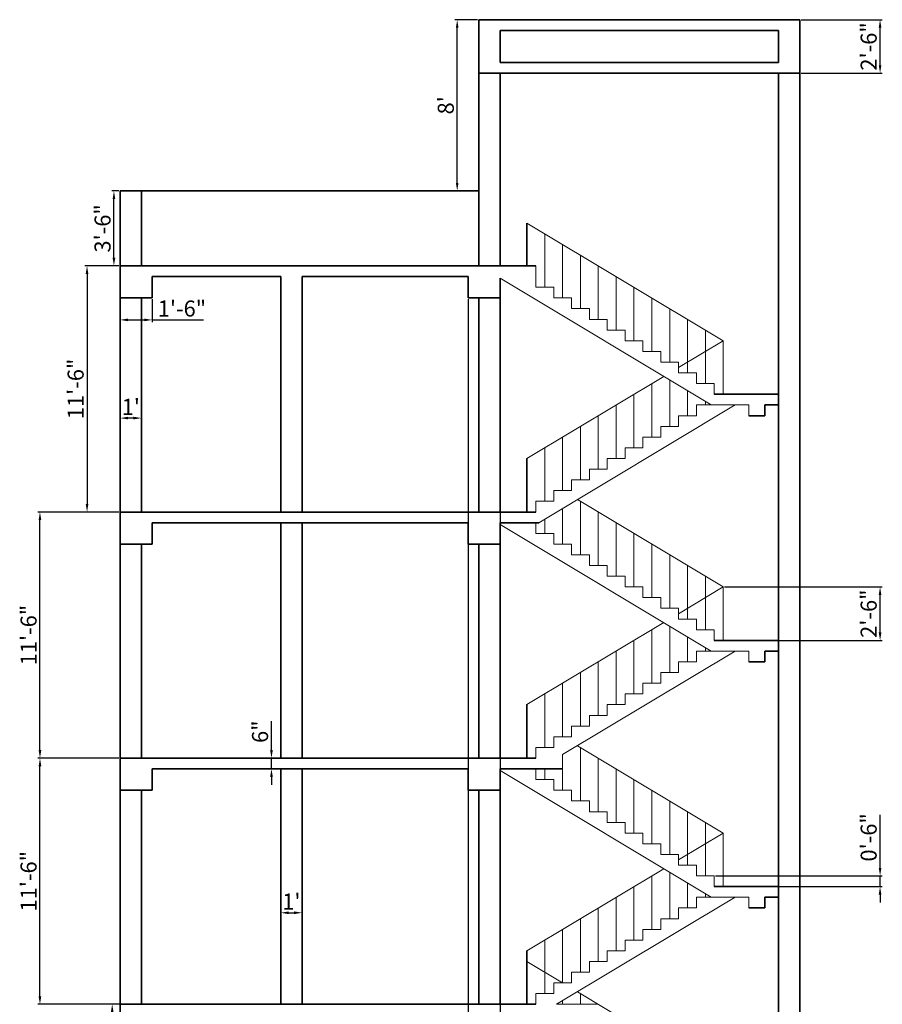
# Model space of a CAD drawing. Units: inches. Extents: x 1692 to 2762, y 798 to 1757.
# Tile 4 of 4: x 2279 to 2762, y 1156 to 1708. Entities that reach past the tile are written whole.
import ezdxf

# ---------------------------------------------------------------- set-up
doc = ezdxf.new("R2010")
doc.units = ezdxf.units.IN
for name, color, linetype, lineweight in [('A-ANNO-DIMS', 2, 'Continuous', 18), ('A-FLOR-STRS', 3, 'Continuous', 18), ('A-SECT', 1, 'Continuous', 35)]:
    doc.layers.add(name, color=color, linetype=linetype, lineweight=lineweight)
doc.styles.get("Standard").update_dxf_attribs({"font": 'arial.ttf'})
doc.dimstyles.new('ISO-25', dxfattribs={"dimtxt": 9, "dimasz": 4.5, "dimexe": 1.25, "dimexo": 0.625, "dimtad": 1, "dimdec": 0, "dimlunit": 3, "dimtxsty": 'Standard', "dimcen": 2.5, "dimadec": 0, "dimazin": 0, "dimtfac": 1, "dimtdec": 0, "dimtmove": 0, "dimatfit": 3, "dimfxl": 1, "dimarcsym": 0})

# ---------------------------------------------------------------- blocks, each defined once
blk = doc.blocks.new('*D1')
at = {"layer": 'A-ANNO-DIMS', "color": 0, "lineweight": -2, "transparency": 16777216}
for p, q in [((2334.16, 1570.43), (2315.01, 1570.43)), ((2316.26, 1565.93), (2316.26, 1436.93)), ((2334.16, 1432.43), (2315.01, 1432.43))]:
    blk.add_line(p, q, dxfattribs=at)
at = {"layer": 'A-ANNO-DIMS', "color": 0, "lineweight": 0, "transparency": 16777216}
for points in [[(2315.51, 1565.93), (2317.01, 1565.93), (2316.26, 1570.43)], [(2315.51, 1436.93), (2317.01, 1436.93), (2316.26, 1432.43)]]:
    blk.add_solid(points, dxfattribs=at)
at = {"layer": 'Defpoints', "color": 0, "lineweight": 0, "transparency": 16777216}
for p in [(2334.78, 1570.43), (2316.26, 1432.43), (2334.78, 1432.43)]:
    blk.add_point(p, dxfattribs=at)
at = {"layer": 'A-ANNO-DIMS', "color": 0, "transparency": 16777216, "insert": (2311.04, 1501.43), "char_height": 9, "attachment_point": 5, "rotation": 90}
blk.add_mtext('11\'-6"', dxfattribs=at)
blk = doc.blocks.new('*D2')
at = {"layer": 'A-ANNO-DIMS', "color": 0, "lineweight": -2, "transparency": 16777216}
for p, q in [((2334.78, 1551.81), (2334.78, 1538.88)), ((2352.78, 1551.81), (2352.78, 1538.88)), ((2339.28, 1540.13), (2348.28, 1540.13)), ((2352.78, 1540.13), (2381.61, 1540.13))]:
    blk.add_line(p, q, dxfattribs=at)
at = {"layer": 'A-ANNO-DIMS', "color": 0, "lineweight": 0, "transparency": 16777216}
for points in [[(2339.28, 1540.88), (2339.28, 1539.38), (2334.78, 1540.13)], [(2348.28, 1540.88), (2348.28, 1539.38), (2352.78, 1540.13)]]:
    blk.add_solid(points, dxfattribs=at)
at = {"layer": 'Defpoints', "color": 0, "lineweight": 0, "transparency": 16777216}
for p in [(2334.78, 1552.43), (2352.78, 1552.43), (2352.78, 1540.13)]:
    blk.add_point(p, dxfattribs=at)
at = {"layer": 'A-ANNO-DIMS', "color": 0, "transparency": 16777216, "insert": (2369.44, 1545.35), "char_height": 9, "attachment_point": 5}
blk.add_mtext('1\'-6"', dxfattribs=at)
blk = doc.blocks.new('*D3')
at = {"layer": 'A-ANNO-DIMS', "color": 0, "lineweight": -2, "transparency": 16777216}
for p, q in [((2334.78, 1478.04), (2334.78, 1486.33)), ((2342.28, 1485.08), (2339.28, 1485.08)), ((2346.78, 1478.04), (2346.78, 1486.33))]:
    blk.add_line(p, q, dxfattribs=at)
at = {"layer": 'A-ANNO-DIMS', "color": 0, "lineweight": 0, "transparency": 16777216}
for points in [[(2339.28, 1485.83), (2339.28, 1484.33), (2334.78, 1485.08)], [(2342.28, 1485.83), (2342.28, 1484.33), (2346.78, 1485.08)]]:
    blk.add_solid(points, dxfattribs=at)
at = {"layer": 'Defpoints', "color": 0, "lineweight": 0, "transparency": 16777216}
for p in [(2334.78, 1485.08), (2334.78, 1477.42), (2346.78, 1477.42)]:
    blk.add_point(p, dxfattribs=at)
at = {"layer": 'A-ANNO-DIMS', "color": 0, "transparency": 16777216, "insert": (2340.78, 1490.22), "char_height": 9, "attachment_point": 5}
blk.add_mtext("1'", dxfattribs=at)
blk = doc.blocks.new('*D5')
at = {"layer": 'A-ANNO-DIMS', "color": 0, "lineweight": -2, "transparency": 16777216}
for p, q in [((2346.16, 1156.43), (2329.11, 1156.43)), ((2330.36, 1151.93), (2330.36, 1142.93)), ((2346.16, 1138.43), (2329.11, 1138.43)), ((2330.36, 1138.43), (2330.36, 1109.61))]:
    blk.add_line(p, q, dxfattribs=at)
at = {"layer": 'A-ANNO-DIMS', "color": 0, "lineweight": 0, "transparency": 16777216}
for points in [[(2329.61, 1151.93), (2331.11, 1151.93), (2330.36, 1156.43)], [(2329.61, 1142.93), (2331.11, 1142.93), (2330.36, 1138.43)]]:
    blk.add_solid(points, dxfattribs=at)
at = {"layer": 'Defpoints', "color": 0, "lineweight": 0, "transparency": 16777216}
for p in [(2346.78, 1156.43), (2330.36, 1138.43), (2346.78, 1138.43)]:
    blk.add_point(p, dxfattribs=at)
at = {"layer": 'A-ANNO-DIMS', "color": 0, "transparency": 16777216, "insert": (2325.14, 1121.77), "char_height": 9, "attachment_point": 5, "rotation": 90}
blk.add_mtext('1\'-6"', dxfattribs=at)
blk = doc.blocks.new('*D7')
at = {"layer": 'A-ANNO-DIMS', "color": 0, "lineweight": -2, "transparency": 16777216}
for p, q in [((2424.78, 1195.02), (2424.78, 1209.01)), ((2436.78, 1195.02), (2436.78, 1209.01)), ((2429.28, 1207.76), (2432.28, 1207.76))]:
    blk.add_line(p, q, dxfattribs=at)
at = {"layer": 'A-ANNO-DIMS', "color": 0, "lineweight": 0, "transparency": 16777216}
for points in [[(2429.28, 1208.51), (2429.28, 1207.01), (2424.78, 1207.76)], [(2432.28, 1208.51), (2432.28, 1207.01), (2436.78, 1207.76)]]:
    blk.add_solid(points, dxfattribs=at)
at = {"layer": 'Defpoints', "color": 0, "lineweight": 0, "transparency": 16777216}
for p in [(2436.78, 1207.76), (2424.78, 1194.4), (2436.78, 1194.4)]:
    blk.add_point(p, dxfattribs=at)
at = {"layer": 'A-ANNO-DIMS', "color": 0, "transparency": 16777216, "insert": (2430.78, 1212.9), "char_height": 9, "attachment_point": 5}
blk.add_mtext("1'", dxfattribs=at)
blk = doc.blocks.new('*D8')
at = {"layer": 'A-ANNO-DIMS', "color": 0, "lineweight": -2, "transparency": 16777216}
for p, q in [((2419.61, 1298.93), (2419.61, 1315.08)), ((2417.71, 1294.43), (2420.86, 1294.43)), ((2419.61, 1288.43), (2419.61, 1294.43)), ((2417.71, 1288.43), (2420.86, 1288.43)), ((2419.61, 1283.93), (2419.61, 1279.43))]:
    blk.add_line(p, q, dxfattribs=at)
at = {"layer": 'A-ANNO-DIMS', "color": 0, "lineweight": 0, "transparency": 16777216}
for points in [[(2418.86, 1298.93), (2420.36, 1298.93), (2419.61, 1294.43)], [(2418.86, 1283.93), (2420.36, 1283.93), (2419.61, 1288.43)]]:
    blk.add_solid(points, dxfattribs=at)
at = {"layer": 'Defpoints', "color": 0, "lineweight": 0, "transparency": 16777216}
for p in [(2417.08, 1294.43), (2419.61, 1294.43), (2417.08, 1288.43)]:
    blk.add_point(p, dxfattribs=at)
at = {"layer": 'A-ANNO-DIMS', "color": 0, "transparency": 16777216, "insert": (2414.39, 1309.25), "char_height": 9, "attachment_point": 5, "rotation": 90}
blk.add_mtext('6"', dxfattribs=at)
blk = doc.blocks.new('*D9')
at = {"layer": 'A-ANNO-DIMS', "color": 0, "lineweight": -2, "transparency": 16777216}
for p, q in [((2334.16, 1612.43), (2330.09, 1612.43)), ((2331.34, 1574.93), (2331.34, 1607.93)), ((2334.16, 1570.43), (2330.09, 1570.43))]:
    blk.add_line(p, q, dxfattribs=at)
at = {"layer": 'A-ANNO-DIMS', "color": 0, "lineweight": 0, "transparency": 16777216}
for points in [[(2330.59, 1607.93), (2332.09, 1607.93), (2331.34, 1612.43)], [(2330.59, 1574.93), (2332.09, 1574.93), (2331.34, 1570.43)]]:
    blk.add_solid(points, dxfattribs=at)
at = {"layer": 'Defpoints', "color": 0, "lineweight": 0, "transparency": 16777216}
for p in [(2331.34, 1612.43), (2334.78, 1612.43), (2334.78, 1570.43)]:
    blk.add_point(p, dxfattribs=at)
at = {"layer": 'A-ANNO-DIMS', "color": 0, "transparency": 16777216, "insert": (2326.12, 1591.43), "char_height": 9, "attachment_point": 5, "rotation": 90}
blk.add_mtext('3\'-6"', dxfattribs=at)
blk = doc.blocks.new('*D10')
at = {"layer": 'A-ANNO-DIMS', "color": 0, "lineweight": -2, "transparency": 16777216}
for p, q in [((2535.16, 1708.43), (2522.45, 1708.43)), ((2523.7, 1616.93), (2523.7, 1703.93)), ((2535.16, 1612.43), (2522.45, 1612.43))]:
    blk.add_line(p, q, dxfattribs=at)
at = {"layer": 'A-ANNO-DIMS', "color": 0, "lineweight": 0, "transparency": 16777216}
for points in [[(2522.95, 1703.93), (2524.45, 1703.93), (2523.7, 1708.43)], [(2522.95, 1616.93), (2524.45, 1616.93), (2523.7, 1612.43)]]:
    blk.add_solid(points, dxfattribs=at)
at = {"layer": 'Defpoints', "color": 0, "lineweight": 0, "transparency": 16777216}
for p in [(2523.7, 1708.43), (2535.78, 1708.43), (2535.78, 1612.43)]:
    blk.add_point(p, dxfattribs=at)
at = {"layer": 'A-ANNO-DIMS', "color": 0, "transparency": 16777216, "insert": (2518.48, 1660.43), "char_height": 9, "attachment_point": 5, "rotation": 90}
blk.add_mtext("8'", dxfattribs=at)
blk = doc.blocks.new('*D54')
at = {"layer": 'A-ANNO-DIMS', "color": 0, "lineweight": -2, "transparency": 16777216}
for p, q in [((2334.16, 1294.43), (2288.63, 1294.43)), ((2289.88, 1160.93), (2289.88, 1289.93)), ((2334.16, 1156.43), (2288.63, 1156.43))]:
    blk.add_line(p, q, dxfattribs=at)
at = {"layer": 'A-ANNO-DIMS', "color": 0, "lineweight": 0, "transparency": 16777216}
for points in [[(2289.13, 1289.93), (2290.63, 1289.93), (2289.88, 1294.43)], [(2289.13, 1160.93), (2290.63, 1160.93), (2289.88, 1156.43)]]:
    blk.add_solid(points, dxfattribs=at)
at = {"layer": 'Defpoints', "color": 0, "lineweight": 0, "transparency": 16777216}
for p in [(2289.88, 1294.43), (2334.78, 1294.43), (2334.78, 1156.43)]:
    blk.add_point(p, dxfattribs=at)
at = {"layer": 'A-ANNO-DIMS', "color": 0, "transparency": 16777216, "insert": (2284.66, 1225.43), "char_height": 9, "attachment_point": 5, "rotation": 90}
blk.add_mtext('11\'-6"', dxfattribs=at)
blk = doc.blocks.new('*D55')
at = {"layer": 'A-ANNO-DIMS', "color": 0, "lineweight": -2, "transparency": 16777216}
for p, q in [((2334.16, 1432.43), (2288.63, 1432.43)), ((2289.88, 1298.93), (2289.88, 1427.93)), ((2334.16, 1294.43), (2288.63, 1294.43))]:
    blk.add_line(p, q, dxfattribs=at)
at = {"layer": 'A-ANNO-DIMS', "color": 0, "lineweight": 0, "transparency": 16777216}
for points in [[(2289.13, 1427.93), (2290.63, 1427.93), (2289.88, 1432.43)], [(2289.13, 1298.93), (2290.63, 1298.93), (2289.88, 1294.43)]]:
    blk.add_solid(points, dxfattribs=at)
at = {"layer": 'Defpoints', "color": 0, "lineweight": 0, "transparency": 16777216}
for p in [(2289.88, 1432.43), (2334.78, 1432.43), (2334.78, 1294.43)]:
    blk.add_point(p, dxfattribs=at)
at = {"layer": 'A-ANNO-DIMS', "color": 0, "transparency": 16777216, "insert": (2284.66, 1363.43), "char_height": 9, "attachment_point": 5, "rotation": 90}
blk.add_mtext('11\'-6"', dxfattribs=at)
blk = doc.blocks.new('*D56')
at = {"layer": 'A-ANNO-DIMS', "color": 0, "lineweight": -2, "transparency": 16777216}
for p, q in [((2716.41, 1708.43), (2761.93, 1708.43)), ((2760.68, 1682.93), (2760.68, 1703.93)), ((2716.41, 1678.43), (2761.93, 1678.43))]:
    blk.add_line(p, q, dxfattribs=at)
at = {"layer": 'A-ANNO-DIMS', "color": 0, "lineweight": 0, "transparency": 16777216}
for points in [[(2759.93, 1703.93), (2761.43, 1703.93), (2760.68, 1708.43)], [(2759.93, 1682.93), (2761.43, 1682.93), (2760.68, 1678.43)]]:
    blk.add_solid(points, dxfattribs=at)
at = {"layer": 'Defpoints', "color": 0, "lineweight": 0, "transparency": 16777216}
for p in [(2715.78, 1708.43), (2760.68, 1708.43), (2715.78, 1678.43)]:
    blk.add_point(p, dxfattribs=at)
at = {"layer": 'A-ANNO-DIMS', "color": 0, "transparency": 16777216, "insert": (2755.46, 1693.43), "char_height": 9, "attachment_point": 5, "rotation": 90}
blk.add_mtext('2\'-6"', dxfattribs=at)
blk = doc.blocks.new('*D65')
at = {"layer": 'A-ANNO-DIMS', "color": 0, "lineweight": -2, "transparency": 16777216}
for p, q in [((2529.78, 1551.81), (2529.78, 798.28)), ((2547.78, 1551.81), (2547.78, 798.28)), ((2534.28, 799.53), (2543.28, 799.53)), ((2547.78, 799.53), (2576.61, 799.53))]:
    blk.add_line(p, q, dxfattribs=at)
at = {"layer": 'A-ANNO-DIMS', "color": 0, "lineweight": 0, "transparency": 16777216}
for points in [[(2534.28, 800.28), (2534.28, 798.78), (2529.78, 799.53)], [(2543.28, 800.28), (2543.28, 798.78), (2547.78, 799.53)]]:
    blk.add_solid(points, dxfattribs=at)
at = {"layer": 'Defpoints', "color": 0, "lineweight": 0, "transparency": 16777216}
for p in [(2529.78, 1552.43), (2547.78, 1552.43), (2547.78, 799.53)]:
    blk.add_point(p, dxfattribs=at)
at = {"layer": 'A-ANNO-DIMS', "color": 0, "transparency": 16777216, "insert": (2564.44, 804.75), "char_height": 9, "attachment_point": 5}
blk.add_mtext('1\'-6"', dxfattribs=at)
blk = doc.blocks.new('*D67')
at = {"layer": 'A-ANNO-DIMS', "color": 0, "lineweight": -2, "transparency": 16777216}
for p, q in [((2760.68, 1232.93), (2760.68, 1262.61)), ((2668.41, 1228.43), (2761.93, 1228.43)), ((2760.68, 1222.43), (2760.68, 1228.43)), ((2668.41, 1222.43), (2761.93, 1222.43)), ((2760.68, 1217.93), (2760.68, 1213.43))]:
    blk.add_line(p, q, dxfattribs=at)
at = {"layer": 'A-ANNO-DIMS', "color": 0, "lineweight": 0, "transparency": 16777216}
for points in [[(2759.93, 1232.93), (2761.43, 1232.93), (2760.68, 1228.43)], [(2759.93, 1217.93), (2761.43, 1217.93), (2760.68, 1222.43)]]:
    blk.add_solid(points, dxfattribs=at)
at = {"layer": 'Defpoints', "color": 0, "lineweight": 0, "transparency": 16777216}
for p in [(2667.78, 1228.43), (2760.68, 1228.43), (2667.78, 1222.43)]:
    blk.add_point(p, dxfattribs=at)
at = {"layer": 'A-ANNO-DIMS', "color": 0, "transparency": 16777216, "insert": (2755.46, 1250.02), "char_height": 9, "attachment_point": 5, "rotation": 90}
blk.add_mtext('0\'-6"', dxfattribs=at)
blk = doc.blocks.new('*D68')
at = {"layer": 'A-ANNO-DIMS', "color": 0, "lineweight": -2, "transparency": 16777216}
for p, q in [((2673.41, 1390.43), (2761.93, 1390.43)), ((2760.68, 1364.93), (2760.68, 1385.93)), ((2673.41, 1360.43), (2761.93, 1360.43))]:
    blk.add_line(p, q, dxfattribs=at)
at = {"layer": 'A-ANNO-DIMS', "color": 0, "lineweight": 0, "transparency": 16777216}
for points in [[(2759.93, 1385.93), (2761.43, 1385.93), (2760.68, 1390.43)], [(2759.93, 1364.93), (2761.43, 1364.93), (2760.68, 1360.43)]]:
    blk.add_solid(points, dxfattribs=at)
at = {"layer": 'Defpoints', "color": 0, "lineweight": 0, "transparency": 16777216}
for p in [(2672.78, 1390.43), (2760.68, 1390.43), (2672.78, 1360.43)]:
    blk.add_point(p, dxfattribs=at)
at = {"layer": 'A-ANNO-DIMS', "color": 0, "transparency": 16777216, "insert": (2755.46, 1375.43), "char_height": 9, "attachment_point": 5, "rotation": 90}
blk.add_mtext('2\'-6"', dxfattribs=at)

msp = doc.modelspace()

# ---------------------------------------------------------------- linework, layer by layer
at = {"layer": 'A-FLOR-STRS'}
for p, q in [((2562.78, 1594.43), (2672.78, 1528.43)), ((2572.78, 1558.43), (2572.78, 1588.43)), ((2582.78, 1552.43), (2582.78, 1582.43)), ((2592.78, 1546.43), (2592.78, 1576.43)), ((2567.78, 1558.43), (2567.78, 1570.43)), ((2602.78, 1540.43), (2602.78, 1570.43)), ((2666.12, 1492.43), (2547.78, 1563.44)), ((2612.78, 1534.43), (2612.78, 1564.43)), ((2577.78, 1558.43), (2567.78, 1558.43)), ((2577.78, 1552.43), (2577.78, 1558.43)), ((2622.78, 1528.43), (2622.78, 1558.43)), ((2587.78, 1552.43), (2577.78, 1552.43)), ((2587.78, 1546.43), (2587.78, 1552.43)), ((2632.78, 1522.43), (2632.78, 1552.43)), ((2597.78, 1546.43), (2587.78, 1546.43)), ((2597.78, 1540.43), (2597.78, 1546.43)), ((2642.78, 1516.43), (2642.78, 1546.43)), ((2607.78, 1540.43), (2597.78, 1540.43)), ((2607.78, 1534.43), (2607.78, 1540.43)), ((2652.78, 1510.43), (2652.78, 1540.43)), ((2617.78, 1534.43), (2607.78, 1534.43)), ((2617.78, 1528.43), (2617.78, 1534.43)), ((2662.78, 1504.43), (2662.78, 1534.43)), ((2627.78, 1528.43), (2617.78, 1528.43)), ((2627.78, 1522.43), (2627.78, 1528.43)), ((2672.78, 1528.43), (2647.78, 1513.43)), ((2672.78, 1498.43), (2672.78, 1528.43)), ((2672.78, 1504.43), (2672.78, 1528.43)), ((2637.78, 1522.43), (2627.78, 1522.43)), ((2637.78, 1516.43), (2637.78, 1522.43)), ((2662.78, 1504.43), (2662.78, 1522.43)), ((2647.78, 1516.43), (2637.78, 1516.43)), ((2647.78, 1510.43), (2647.78, 1516.43)), ((2652.78, 1510.43), (2652.78, 1516.43)), ((2639.45, 1508.43), (2562.78, 1462.43)), ((2657.78, 1510.43), (2647.78, 1510.43)), ((2657.78, 1504.43), (2657.78, 1510.43)), ((2632.78, 1474.43), (2632.78, 1504.43)), ((2642.78, 1480.43), (2642.78, 1506.44)), ((2667.78, 1504.43), (2657.78, 1504.43)), ((2667.78, 1498.43), (2667.78, 1504.43)), ((2672.78, 1498.43), (2672.78, 1504.43)), ((2622.78, 1468.43), (2622.78, 1498.43)), ((2652.78, 1486.43), (2652.78, 1500.44)), ((2679.44, 1492.43), (2569.44, 1426.43)), ((2612.78, 1462.43), (2612.78, 1492.43)), ((2657.78, 1486.43), (2657.78, 1492.43)), ((2657.78, 1492.43), (2679.44, 1492.43)), ((2662.78, 1492.43), (2662.78, 1494.44)), ((2679.44, 1492.43), (2687.11, 1492.43)), ((2687.11, 1492.43), (2687.11, 1486.43)), ((2602.78, 1456.43), (2602.78, 1486.43)), ((2647.78, 1480.43), (2647.78, 1486.43)), ((2647.78, 1486.43), (2657.78, 1486.43)), ((2592.78, 1450.43), (2592.78, 1480.43)), ((2637.78, 1474.43), (2637.78, 1480.43)), ((2637.78, 1480.43), (2647.78, 1480.43)), ((2582.78, 1444.43), (2582.78, 1474.43)), ((2627.78, 1468.43), (2627.78, 1474.43)), ((2627.78, 1474.43), (2637.78, 1474.43)), ((2572.78, 1438.43), (2572.78, 1468.43)), ((2617.78, 1462.43), (2617.78, 1468.43)), ((2617.78, 1468.43), (2627.78, 1468.43)), ((2607.78, 1456.43), (2607.78, 1462.43)), ((2607.78, 1462.43), (2617.78, 1462.43)), ((2597.78, 1450.43), (2597.78, 1456.43)), ((2597.78, 1456.43), (2607.78, 1456.43)), ((2572.78, 1438.43), (2572.78, 1450.43)), ((2587.78, 1444.43), (2587.78, 1450.43)), ((2587.78, 1450.43), (2597.78, 1450.43)), ((2577.78, 1438.43), (2577.78, 1444.43)), ((2577.78, 1444.43), (2587.78, 1444.43)), ((2567.78, 1432.43), (2567.78, 1438.43)), ((2567.78, 1438.43), (2577.78, 1438.43)), ((2591.11, 1439.43), (2672.78, 1390.43)), ((2592.78, 1408.43), (2592.78, 1438.43)), ((2582.78, 1414.43), (2582.78, 1434.44)), ((2602.78, 1402.43), (2602.78, 1432.43)), ((2666.12, 1354.43), (2547.78, 1425.44)), ((2567.78, 1426.43), (2569.44, 1426.43)), ((2567.78, 1420.43), (2567.78, 1426.43)), ((2567.78, 1420.43), (2567.78, 1426.43)), ((2572.78, 1420.43), (2572.78, 1428.44)), ((2612.78, 1396.43), (2612.78, 1426.43)), ((2577.78, 1420.43), (2567.78, 1420.43)), ((2577.78, 1414.43), (2577.78, 1420.43)), ((2622.78, 1390.43), (2622.78, 1420.43)), ((2587.78, 1414.43), (2577.78, 1414.43)), ((2587.78, 1408.43), (2587.78, 1414.43)), ((2632.78, 1384.43), (2632.78, 1414.43)), ((2597.78, 1408.43), (2587.78, 1408.43)), ((2597.78, 1402.43), (2597.78, 1408.43)), ((2642.78, 1378.43), (2642.78, 1408.43)), ((2607.78, 1402.43), (2597.78, 1402.43)), ((2607.78, 1396.43), (2607.78, 1402.43)), ((2652.78, 1372.43), (2652.78, 1402.43)), ((2617.78, 1396.43), (2607.78, 1396.43)), ((2617.78, 1390.43), (2617.78, 1396.43)), ((2662.78, 1366.43), (2662.78, 1396.43)), ((2627.78, 1390.43), (2617.78, 1390.43)), ((2627.78, 1384.43), (2627.78, 1390.43)), ((2672.78, 1390.43), (2647.78, 1375.43)), ((2672.78, 1360.43), (2672.78, 1390.43)), ((2672.78, 1366.43), (2672.78, 1390.43)), ((2637.78, 1384.43), (2627.78, 1384.43)), ((2637.78, 1378.43), (2637.78, 1384.43)), ((2662.78, 1366.43), (2662.78, 1384.43)), ((2647.78, 1378.43), (2637.78, 1378.43)), ((2647.78, 1372.43), (2647.78, 1378.43)), ((2652.78, 1372.43), (2652.78, 1378.43)), ((2639.45, 1370.43), (2562.78, 1324.43)), ((2657.78, 1372.43), (2647.78, 1372.43)), ((2657.78, 1366.43), (2657.78, 1372.43)), ((2632.78, 1336.43), (2632.78, 1366.43)), ((2642.78, 1342.43), (2642.78, 1368.44)), ((2667.78, 1366.43), (2657.78, 1366.43)), ((2667.78, 1360.43), (2667.78, 1366.43)), ((2672.78, 1360.43), (2672.78, 1366.43)), ((2622.78, 1330.43), (2622.78, 1360.43)), ((2652.78, 1348.43), (2652.78, 1362.44)), ((2582.78, 1296.44), (2679.44, 1354.43)), ((2612.78, 1324.43), (2612.78, 1354.43)), ((2657.78, 1348.43), (2657.78, 1354.43)), ((2657.78, 1354.43), (2667.78, 1354.43)), ((2662.78, 1354.43), (2662.78, 1356.44)), ((2667.78, 1354.43), (2687.11, 1354.43)), ((2687.11, 1354.43), (2687.11, 1348.43)), ((2602.78, 1318.43), (2602.78, 1348.43)), ((2647.78, 1342.43), (2647.78, 1348.43)), ((2647.78, 1348.43), (2657.78, 1348.43)), ((2592.78, 1312.43), (2592.78, 1342.43)), ((2637.78, 1336.43), (2637.78, 1342.43)), ((2637.78, 1342.43), (2647.78, 1342.43)), ((2582.78, 1306.43), (2582.78, 1336.43)), ((2627.78, 1330.43), (2627.78, 1336.43)), ((2627.78, 1336.43), (2637.78, 1336.43)), ((2572.78, 1300.43), (2572.78, 1330.43)), ((2617.78, 1324.43), (2617.78, 1330.43)), ((2617.78, 1330.43), (2627.78, 1330.43)), ((2607.78, 1318.43), (2607.78, 1324.43)), ((2607.78, 1324.43), (2617.78, 1324.43)), ((2597.78, 1312.43), (2597.78, 1318.43)), ((2597.78, 1318.43), (2607.78, 1318.43)), ((2572.78, 1300.43), (2572.78, 1312.43)), ((2587.78, 1306.43), (2587.78, 1312.43)), ((2587.78, 1312.43), (2597.78, 1312.43)), ((2577.78, 1300.43), (2577.78, 1306.43)), ((2577.78, 1306.43), (2587.78, 1306.43)), ((2567.78, 1300.43), (2577.78, 1300.43)), ((2567.78, 1294.43), (2567.78, 1300.43)), ((2591.11, 1301.43), (2672.78, 1252.43)), ((2592.78, 1294.43), (2592.78, 1300.43)), ((2582.78, 1294.43), (2582.78, 1296.44)), ((2582.78, 1276.43), (2582.78, 1294.43)), ((2592.78, 1270.43), (2592.78, 1294.43)), ((2602.78, 1264.43), (2602.78, 1294.43)), ((2666.12, 1216.43), (2547.78, 1287.44)), ((2567.78, 1282.43), (2567.78, 1288.43)), ((2567.78, 1282.43), (2567.78, 1288.43)), ((2572.78, 1282.43), (2572.78, 1288.43)), ((2612.78, 1258.43), (2612.78, 1288.43)), ((2577.78, 1282.43), (2567.78, 1282.43)), ((2577.78, 1276.43), (2577.78, 1282.43)), ((2622.78, 1252.43), (2622.78, 1282.43)), ((2587.78, 1276.43), (2577.78, 1276.43)), ((2587.78, 1270.43), (2587.78, 1276.43)), ((2632.78, 1246.43), (2632.78, 1276.43)), ((2597.78, 1270.43), (2587.78, 1270.43)), ((2597.78, 1264.43), (2597.78, 1270.43)), ((2642.78, 1240.43), (2642.78, 1270.43)), ((2607.78, 1264.43), (2597.78, 1264.43)), ((2607.78, 1258.43), (2607.78, 1264.43)), ((2652.78, 1234.43), (2652.78, 1264.43)), ((2617.78, 1258.43), (2607.78, 1258.43)), ((2617.78, 1252.43), (2617.78, 1258.43)), ((2662.78, 1228.43), (2662.78, 1258.43)), ((2627.78, 1252.43), (2617.78, 1252.43)), ((2627.78, 1246.43), (2627.78, 1252.43)), ((2672.78, 1252.43), (2647.78, 1237.43)), ((2672.78, 1222.43), (2672.78, 1252.43)), ((2672.78, 1252.43), (2672.78, 1240.43)), ((2637.78, 1246.43), (2627.78, 1246.43)), ((2637.78, 1240.43), (2637.78, 1246.43)), ((2662.78, 1228.43), (2662.78, 1246.43)), ((2647.78, 1240.43), (2637.78, 1240.43)), ((2647.78, 1234.43), (2647.78, 1240.43)), ((2652.78, 1234.43), (2652.78, 1240.43)), ((2639.45, 1232.43), (2562.78, 1186.43)), ((2657.78, 1234.43), (2647.78, 1234.43)), ((2657.78, 1228.43), (2657.78, 1234.43)), ((2672.78, 1222.43), (2672.78, 1234.43)), ((2632.78, 1198.43), (2632.78, 1228.43)), ((2642.78, 1204.43), (2642.78, 1230.44)), ((2667.78, 1228.43), (2657.78, 1228.43)), ((2667.78, 1222.43), (2667.78, 1228.43)), ((2672.78, 1222.43), (2672.78, 1228.43)), ((2622.78, 1192.43), (2622.78, 1222.43)), ((2652.78, 1210.43), (2652.78, 1224.44)), ((2672.78, 1222.43), (2672.78, 1223.43)), ((2579.44, 1156.43), (2679.44, 1216.43)), ((2612.78, 1186.43), (2612.78, 1216.43)), ((2657.78, 1210.43), (2657.78, 1216.43)), ((2657.78, 1216.43), (2667.78, 1216.43)), ((2662.78, 1216.43), (2662.78, 1218.44)), ((2667.78, 1216.43), (2687.11, 1216.43)), ((2687.11, 1216.43), (2687.11, 1210.43)), ((2602.78, 1180.43), (2602.78, 1210.43)), ((2647.78, 1204.43), (2647.78, 1210.43)), ((2647.78, 1210.43), (2657.78, 1210.43)), ((2592.78, 1174.43), (2592.78, 1204.43)), ((2637.78, 1198.43), (2637.78, 1204.43)), ((2637.78, 1204.43), (2647.78, 1204.43)), ((2582.78, 1168.43), (2582.78, 1198.43)), ((2627.78, 1192.43), (2627.78, 1198.43)), ((2627.78, 1198.43), (2637.78, 1198.43)), ((2572.78, 1162.43), (2572.78, 1192.43)), ((2617.78, 1186.43), (2617.78, 1192.43)), ((2617.78, 1192.43), (2627.78, 1192.43)), ((2607.78, 1180.43), (2607.78, 1186.43)), ((2607.78, 1186.43), (2617.78, 1186.43)), ((2562.78, 1180.43), (2582.78, 1168.43)), ((2597.78, 1174.43), (2597.78, 1180.43)), ((2597.78, 1180.43), (2607.78, 1180.43)), ((2572.78, 1162.43), (2572.78, 1174.43)), ((2587.78, 1168.43), (2587.78, 1174.43)), ((2587.78, 1174.43), (2597.78, 1174.43)), ((2577.78, 1162.43), (2577.78, 1168.43)), ((2577.78, 1168.43), (2587.78, 1168.43)), ((2567.78, 1162.43), (2577.78, 1162.43)), ((2567.78, 1156.43), (2567.78, 1162.43)), ((2591.11, 1163.43), (2672.78, 1114.43)), ((2592.78, 1156.43), (2592.78, 1162.43)), ((2579.44, 1156.43), (2602.78, 1156.43)), ((2582.78, 1156.43), (2582.78, 1158.44))]:
    msp.add_line(p, q, dxfattribs=at)
at = {"layer": 'A-SECT'}
for p, q in [((2535.78, 1708.43), (2535.78, 1570.43)), ((2535.78, 1708.43), (2715.78, 1708.43)), ((2715.78, 1708.43), (2715.78, 844.43)), ((2547.78, 1702.43), (2547.78, 1684.43)), ((2547.78, 1702.43), (2703.78, 1702.43)), ((2703.78, 1702.43), (2703.78, 1684.43)), ((2547.78, 1684.43), (2703.78, 1684.43)), ((2535.78, 1678.43), (2715.78, 1678.43)), ((2547.78, 1678.43), (2547.78, 1570.43)), ((2703.78, 1678.43), (2703.78, 844.43)), ((2334.78, 1612.43), (2334.78, 844.43)), ((2334.78, 1612.43), (2346.78, 1612.43)), ((2346.78, 1612.43), (2346.78, 1570.43)), ((2346.78, 1612.43), (2535.78, 1612.43)), ((2562.78, 1570.43), (2562.78, 1594.43)), ((2334.78, 1570.43), (2567.78, 1570.43)), ((2352.78, 1564.43), (2424.78, 1564.43)), ((2352.78, 1564.43), (2352.78, 1552.43)), ((2424.78, 1564.43), (2424.78, 1432.43)), ((2436.78, 1564.43), (2436.78, 1432.43)), ((2436.78, 1564.43), (2529.78, 1564.43)), ((2529.78, 1564.43), (2529.78, 1552.43)), ((2547.78, 1563.44), (2547.78, 1432.43)), ((2334.78, 1552.43), (2352.78, 1552.43)), ((2346.78, 1552.43), (2346.78, 1432.43)), ((2529.78, 1552.43), (2547.78, 1552.43)), ((2535.78, 1552.43), (2535.78, 1432.43)), ((2667.78, 1498.43), (2703.78, 1498.43)), ((2696.11, 1492.43), (2696.11, 1486.43)), ((2696.11, 1492.43), (2703.78, 1492.43)), ((2687.11, 1486.43), (2696.11, 1486.43)), ((2562.78, 1432.43), (2562.78, 1462.43)), ((2562.78, 1432.43), (2562.78, 1456.43)), ((2334.78, 1432.43), (2567.78, 1432.43)), ((2352.78, 1426.43), (2529.78, 1426.43)), ((2352.78, 1426.43), (2352.78, 1414.43)), ((2424.78, 1426.43), (2424.78, 1294.43)), ((2436.78, 1426.43), (2436.78, 1294.43)), ((2529.78, 1426.43), (2529.78, 1414.43)), ((2547.78, 1426.43), (2547.78, 1294.43)), ((2569.44, 1426.43), (2547.78, 1426.43)), ((2334.78, 1414.43), (2352.78, 1414.43)), ((2346.78, 1414.43), (2346.78, 1294.43)), ((2529.78, 1414.43), (2547.78, 1414.43)), ((2535.78, 1414.43), (2535.78, 1294.43)), ((2667.78, 1360.43), (2703.78, 1360.43)), ((2696.11, 1354.43), (2696.11, 1348.43)), ((2696.11, 1354.43), (2703.78, 1354.43)), ((2687.11, 1348.43), (2696.11, 1348.43)), ((2562.78, 1294.43), (2562.78, 1324.43)), ((2562.78, 1294.43), (2562.78, 1318.43)), ((2334.78, 1294.43), (2567.78, 1294.43)), ((2352.78, 1288.43), (2352.78, 1276.43)), ((2352.78, 1288.43), (2529.78, 1288.43)), ((2424.78, 1288.43), (2424.78, 1156.43)), ((2436.78, 1288.43), (2436.78, 1156.43)), ((2529.78, 1288.43), (2529.78, 1276.43)), ((2547.78, 1288.43), (2582.78, 1288.43)), ((2547.78, 1288.43), (2547.78, 1156.43)), ((2334.78, 1276.43), (2352.78, 1276.43)), ((2346.78, 1276.43), (2346.78, 1156.43)), ((2529.78, 1276.43), (2547.78, 1276.43)), ((2535.78, 1276.43), (2535.78, 1156.43)), ((2667.78, 1222.43), (2703.78, 1222.43)), ((2696.11, 1216.43), (2696.11, 1210.43)), ((2696.11, 1216.43), (2703.78, 1216.43)), ((2687.11, 1210.43), (2696.11, 1210.43)), ((2562.78, 1156.43), (2562.78, 1186.43)), ((2562.78, 1186.43), (2562.78, 1174.43)), ((2562.78, 1156.43), (2562.78, 1180.43)), ((2562.78, 1156.43), (2562.78, 1168.43)), ((2334.78, 1156.43), (2567.78, 1156.43))]:
    msp.add_line(p, q, dxfattribs=at)

# ---------------------------------------------------------------- dimensions: what is measured, and where the dimension line sits
at = {"layer": 'A-ANNO-DIMS'}
for base, p1, p2, override, picture, middle in [((2523.7, 1708.43), (2535.78, 1612.43), (2535.78, 1708.43), {"dimclrd": 0, "dimclre": 0, "dimclrt": 0}, '*D10', (2518.48, 1660.43)), ((2760.68, 1708.43), (2715.78, 1678.43), (2715.78, 1708.43), {"dimdec": 1, "dimlfac": 1, "dimrnd": 0, "dimzin": 1, "dimdsep": 46, "dimlunit": 4, "dimfrac": 2}, '*D56', (2755.46, 1693.43)), ((2331.34, 1612.43), (2334.78, 1570.43), (2334.78, 1612.43), {"dimclrd": 0, "dimclre": 0, "dimclrt": 0}, '*D9', (2326.12, 1591.43)), ((2316.26, 1432.43), (2334.78, 1570.43), (2334.78, 1432.43), {"dimclrd": 0, "dimclre": 0, "dimclrt": 0}, '*D1', (2311.04, 1501.43)), ((2289.88, 1432.43), (2334.78, 1294.43), (2334.78, 1432.43), {"dimdec": 1, "dimlfac": 1, "dimrnd": 0, "dimzin": 1, "dimdsep": 46, "dimlunit": 4, "dimfrac": 2}, '*D55', (2284.66, 1363.43)), ((2760.68, 1390.43), (2672.78, 1360.43), (2672.78, 1390.43), {"dimdec": 1, "dimlfac": 1, "dimrnd": 0, "dimzin": 1, "dimdsep": 46, "dimlunit": 4, "dimfrac": 2}, '*D68', (2755.46, 1375.43)), ((2419.61, 1294.43), (2417.08, 1288.43), (2417.08, 1294.43), {"dimclrd": 0, "dimclre": 0, "dimclrt": 0}, '*D8', (2414.39, 1309.25)), ((2289.88, 1294.43), (2334.78, 1156.43), (2334.78, 1294.43), {"dimdec": 1, "dimlfac": 1, "dimrnd": 0, "dimzin": 1, "dimdsep": 46, "dimlunit": 4, "dimfrac": 2}, '*D54', (2284.66, 1225.43)), ((2760.68, 1228.43), (2667.78, 1222.43), (2667.78, 1228.43), {"dimdec": 1, "dimlfac": 1, "dimrnd": 0, "dimzin": 1, "dimdsep": 46, "dimlunit": 4, "dimfrac": 2}, '*D67', (2755.46, 1250.02)), ((2330.36, 1138.43), (2346.78, 1156.43), (2346.78, 1138.43), {"dimclrd": 0, "dimclre": 0, "dimclrt": 0}, '*D5', (2325.14, 1121.77))]:
    dim = msp.add_linear_dim(base=base, p1=p1, p2=p2, angle=90, dimstyle='ISO-25', override=override, dxfattribs=at)
    dim.commit()
    dim.dimension.update_dxf_attribs({"geometry": picture, "text_midpoint": middle})
for base, p1, p2, override, picture, middle in [((2352.78, 1540.13), (2334.78, 1552.43), (2352.78, 1552.43), {"dimclrd": 0, "dimclre": 0, "dimclrt": 0}, '*D2', (2369.44, 1545.35)), ((2547.78, 799.53), (2529.78, 1552.43), (2547.78, 1552.43), {"dimdec": 1, "dimlfac": 1, "dimrnd": 0, "dimzin": 1, "dimdsep": 46, "dimlunit": 4, "dimfrac": 2}, '*D65', (2564.44, 804.75)), ((2334.78, 1485.08), (2346.78, 1477.42), (2334.78, 1477.42), {"dimclrd": 0, "dimclre": 0, "dimclrt": 0}, '*D3', (2340.78, 1490.22)), ((2436.78, 1207.76), (2424.78, 1194.4), (2436.78, 1194.4), {"dimclrd": 0, "dimclre": 0, "dimclrt": 0}, '*D7', (2430.78, 1212.9))]:
    dim = msp.add_linear_dim(base=base, p1=p1, p2=p2, dimstyle='ISO-25', override=override, dxfattribs=at)
    dim.commit()
    dim.dimension.update_dxf_attribs({"geometry": picture, "text_midpoint": middle})

doc.saveas('drawing.dxf')
